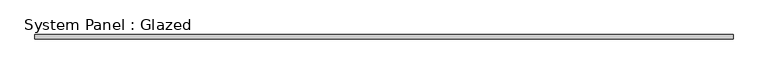
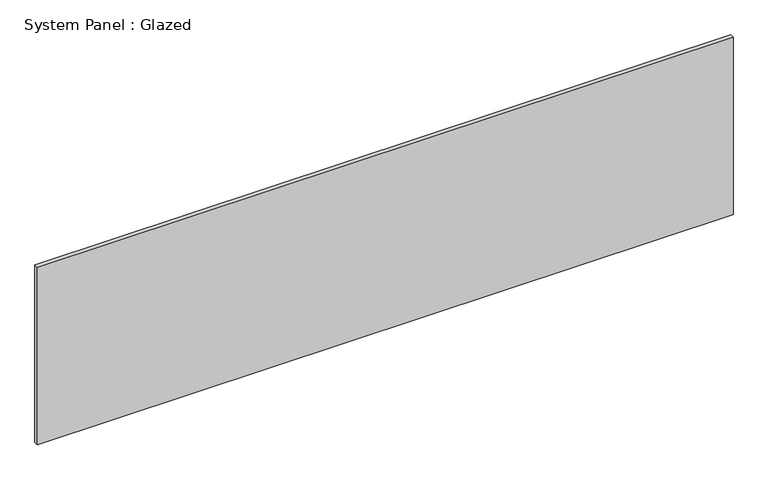
"""IFC4 building model written with IfcOpenShell, lengths in millimetres: plate geometry, System Panel : Glazed."""

from ifc_helpers import new_model, si_unit, origin, origin_with_axes, place, context, project, spatial, polyline, outline, extrude, source, transform, mapped, element, save


def system_panel_glazed_b0cc1a2f(model_context):
    return source(origin(), model_context, "Body", "SweptSolid", [
        extrude(outline(polyline([(2025.65, 19.05), (-2025.65, 19.05), (-2025.65, 44.45), (2025.65, 44.45), (2025.65, 19.05)])), origin_with_axes(), (0.0, 0.0, 1.0), 1092.2),
    ])


if __name__ == "__main__":
    model = new_model("IFC4")
    model_context = context("Model", 3, world=origin())
    ifc_project = project(units=[si_unit("LENGTHUNIT", "METRE", prefix="MILLI")], contexts=[model_context])
    site = spatial("IfcSite", under=ifc_project)
    building = spatial("IfcBuilding", under=site)
    placement = place(None, origin())
    system_panel_glazed_shape = system_panel_glazed_b0cc1a2f(model_context)
    element("IfcPlate", 1, ObjectType="System Panel : Glazed", at=placement, inside=building, context=model_context, shape_type="MappedRepresentation", body=[
        mapped(system_panel_glazed_shape, transform((0.0, 0.0, 0.0), x_axis=(1.0, 0.0, 0.0), y_axis=(0.0, 1.0, 0.0), z_axis=(0.0, 0.0, 1.0))),
    ])
    save(model, "model.ifc")

# Revit data of these elements
# Type "System Panel : Glazed"
#   Construction Type Id = "GSP4R"
#   Analytic Construction = "1/8 in Pilkington single glazing"
#   Visual Light Transmittance = 0.9
#   Solar Heat Gain Coefficient = 0.86
#   Heat Transfer Coefficient (U) = 1.18115 BTU/(h·ft²·°F)
# Element 1 (IfcPlate, "System Panel : Glazed")
#   Materials on its faces: "Glass"
# Materials
#   "Glass": class "Glass", colour RGB 0 128 192, transparency 0.75, Description = "Soda Lime Glass", Cost = 0
